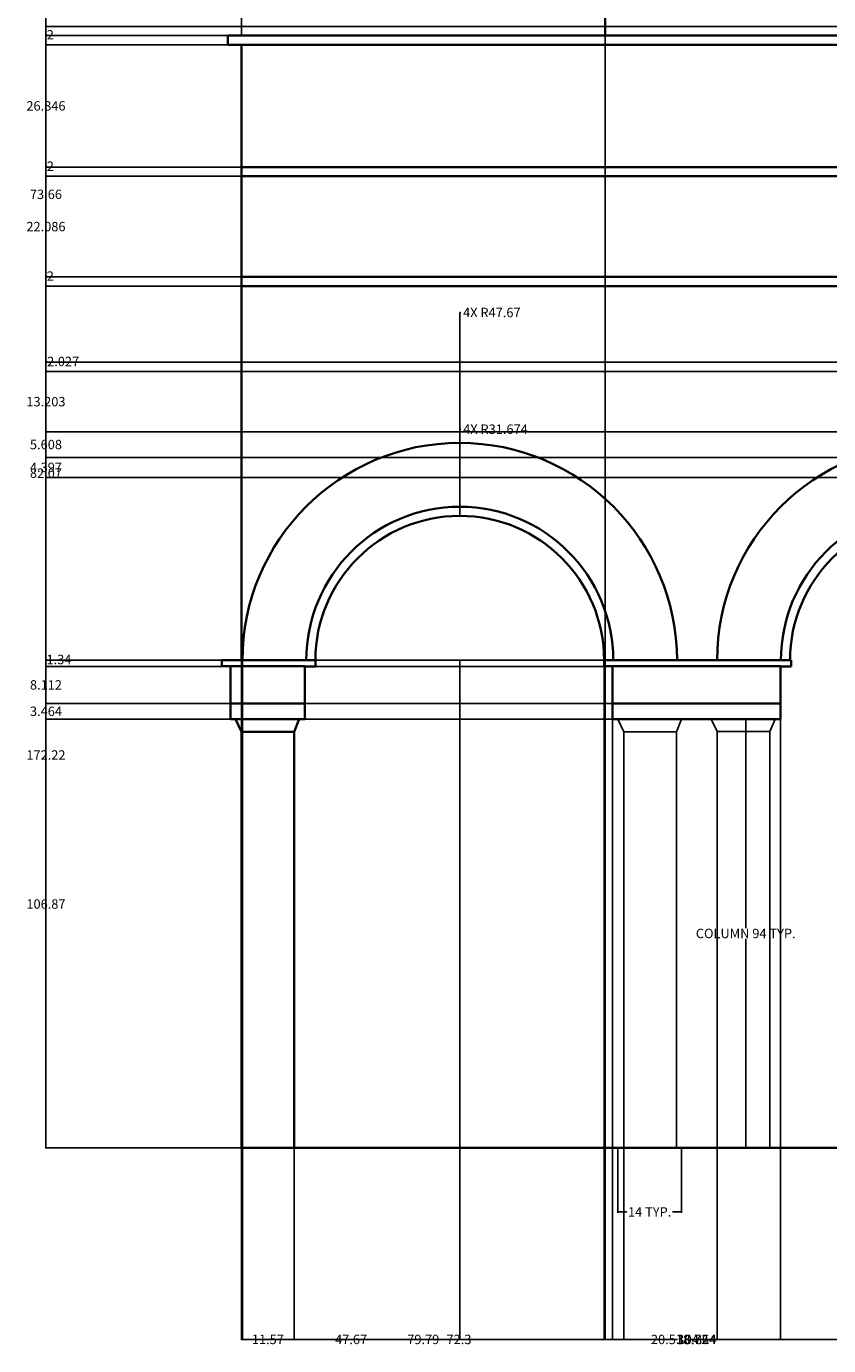
# Model space of a CAD drawing. Units: inches. Extents: x 14 to 859, y 52 to 711.
# Tile 1 of 11: x 14 to 190, y 52 to 342. Entities that reach past the tile are written whole.
import ezdxf

# ---------------------------------------------------------------- set-up
doc = ezdxf.new("R2010")
doc.units = ezdxf.units.IN
doc.header["$MEASUREMENT"] = 0
for name, color, linetype, lineweight in [('A-ANNO-DIMS', 2, 'Continuous', 18), ('A-COLS', 7, 'Continuous', 25), ('A-ELEV', 7, 'Continuous', 35)]:
    doc.layers.add(name, color=color, linetype=linetype, lineweight=lineweight)
doc.styles.get("Standard").update_dxf_attribs({"font": 'arial.ttf'})
doc.dimstyles.get("Standard").update_dxf_attribs({"dimtxt": 2.0625, "dimasz": 0.18, "dimexe": 0.18, "dimexo": 0.0625, "dimgap": 0.09, "dimtad": 0, "dimtih": 1, "dimtoh": 1, "dimdec": 4, "dimzin": 0, "dimdsep": 46, "dimlunit": 4, "dimtxsty": 'Standard', "dimcen": 0.09, "dimadec": 0, "dimazin": 0, "dimtfac": 1, "dimtdec": 4, "dimtofl": 0, "dimtmove": 0, "dimatfit": 3, "dimfxl": 1, "dimtolj": 1, "dimtzin": 0, "dimarcsym": 0})

# ---------------------------------------------------------------- blocks, each defined once
blk = doc.blocks.new('COLUMN')
for p, q in [((1.31, 91.21), (0, 93.94)), ((12.88, 91.21), (13.98, 93.94)), ((1.31, 0), (1.31, 91.21)), ((12.88, 91.21), (1.31, 91.21)), ((12.88, 0), (12.88, 91.21))]:
    blk.add_line(p, q)
blk = doc.blocks.new('*D5')
at = {"layer": 'A-ANNO-DIMS', "color": 0, "lineweight": -2, "transparency": 16777216}
for p, q in [((157.39, 189.73), (171.59, 189.73)), ((171.41, 189.55), (171.41, 143.92)), ((171.41, 95.97), (171.41, 141.6)), ((157.39, 95.79), (171.59, 95.79))]:
    blk.add_line(p, q, dxfattribs=at)
at = {"layer": 'A-ANNO-DIMS', "color": 0, "transparency": 16777216}
for points in [[(171.38, 189.55), (171.44, 189.55), (171.41, 189.73)], [(171.38, 95.97), (171.44, 95.97), (171.41, 95.79)]]:
    blk.add_solid(points, dxfattribs=at)
at = {"layer": 'Defpoints', "color": 0, "transparency": 16777216}
for p in [(157.32, 189.73), (171.41, 189.73), (157.32, 95.79)]:
    blk.add_point(p, dxfattribs=at)
at = {"layer": 'A-ANNO-DIMS', "color": 0, "transparency": 16777216, "insert": (171.41, 142.76), "char_height": 2.0625, "attachment_point": 5}
blk.add_mtext('\\A1;COLUMN 94 TYP.', dxfattribs=at)
blk = doc.blocks.new('*D6')
at = {"layer": 'A-ANNO-DIMS', "color": 0, "lineweight": -2, "transparency": 16777216}
for p, q in [((143.34, 95.73), (143.34, 81.52)), ((157.32, 95.73), (157.32, 81.52)), ((143.52, 81.7), (145.32, 81.7)), ((157.14, 81.7), (155.34, 81.7))]:
    blk.add_line(p, q, dxfattribs=at)
at = {"layer": 'A-ANNO-DIMS', "color": 0, "transparency": 16777216}
for points in [[(143.52, 81.73), (143.52, 81.67), (143.34, 81.7)], [(157.14, 81.73), (157.14, 81.67), (157.32, 81.7)]]:
    blk.add_solid(points, dxfattribs=at)
at = {"layer": 'Defpoints', "color": 0, "transparency": 16777216}
for p in [(143.34, 95.79), (157.32, 95.79), (157.32, 81.7)]:
    blk.add_point(p, dxfattribs=at)
at = {"layer": 'A-ANNO-DIMS', "color": 0, "transparency": 16777216, "insert": (150.33, 81.7), "char_height": 2.0625, "attachment_point": 5}
blk.add_mtext('\\A1;14 TYP.', dxfattribs=at)
blk = doc.blocks.new('*D13')
at = {"layer": 'A-ANNO-DIMS', "color": 0, "lineweight": -2, "transparency": 16777216}
for p, q in [((60.78, 339.73), (60.78, 709.71)), ((60.96, 709.53), (432.6, 709.53)), ((811.37, 709.53), (439.73, 709.53)), ((811.55, 339.73), (811.55, 709.71))]:
    blk.add_line(p, q, dxfattribs=at)
at = {"layer": 'A-ANNO-DIMS', "color": 0, "transparency": 16777216}
for points in [[(60.96, 709.56), (60.96, 709.5), (60.78, 709.53)], [(811.37, 709.56), (811.37, 709.5), (811.55, 709.53)]]:
    blk.add_solid(points, dxfattribs=at)
at = {"layer": 'Defpoints', "color": 0, "transparency": 16777216}
for p in [(811.55, 709.53), (60.78, 339.66), (811.55, 339.66)]:
    blk.add_point(p, dxfattribs=at)
at = {"layer": 'A-ANNO-DIMS', "color": 0, "transparency": 16777216, "insert": (436.17, 709.53), "char_height": 2.062, "attachment_point": 5}
blk.add_mtext('\\A1;750.8', dxfattribs=at)
blk = doc.blocks.new('*D16')
at = {"layer": 'A-ANNO-DIMS', "color": 0, "lineweight": -2, "transparency": 16777216}
for p, q in [((429.96, 670.76), (17.7, 670.76)), ((17.88, 670.58), (17.88, 384.41)), ((17.88, 95.97), (17.88, 382.14)), ((60.72, 95.79), (17.7, 95.79))]:
    blk.add_line(p, q, dxfattribs=at)
at = {"layer": 'A-ANNO-DIMS', "color": 0, "transparency": 16777216}
for points in [[(17.85, 670.58), (17.91, 670.58), (17.88, 670.76)], [(17.85, 95.97), (17.91, 95.97), (17.88, 95.79)]]:
    blk.add_solid(points, dxfattribs=at)
at = {"layer": 'Defpoints', "color": 0, "transparency": 16777216}
for p in [(17.88, 670.76), (430.02, 670.76), (60.78, 95.79)]:
    blk.add_point(p, dxfattribs=at)
at = {"layer": 'A-ANNO-DIMS', "color": 0, "transparency": 16777216, "insert": (17.88, 383.28), "char_height": 2.062, "attachment_point": 5}
blk.add_mtext('\\A1;575', dxfattribs=at)
blk = doc.blocks.new('*D20')
at = {"layer": 'A-ANNO-DIMS', "color": 0, "lineweight": -2, "transparency": 16777216}
for p, q in [((298.67, 268.01), (17.7, 268.01)), ((17.88, 267.83), (17.88, 183.02)), ((17.88, 95.97), (17.88, 180.77)), ((302.61, 95.79), (17.7, 95.79))]:
    blk.add_line(p, q, dxfattribs=at)
at = {"layer": 'A-ANNO-DIMS', "color": 0, "transparency": 16777216}
for points in [[(17.85, 267.83), (17.91, 267.83), (17.88, 268.01)], [(17.85, 95.97), (17.91, 95.97), (17.88, 95.79)]]:
    blk.add_solid(points, dxfattribs=at)
at = {"layer": 'Defpoints', "color": 0, "transparency": 16777216}
for p in [(17.88, 268.01), (298.73, 268.01), (302.67, 95.79)]:
    blk.add_point(p, dxfattribs=at)
at = {"layer": 'A-ANNO-DIMS', "color": 0, "transparency": 16777216, "insert": (17.88, 181.9), "char_height": 2.062, "attachment_point": 5}
blk.add_mtext('\\A1;172.22', dxfattribs=at)
blk = doc.blocks.new('*D25')
at = {"layer": 'A-ANNO-DIMS', "color": 0, "lineweight": -2, "transparency": 16777216}
for p, q in [((298.67, 341.67), (17.7, 341.67)), ((17.88, 341.49), (17.88, 305.98)), ((17.88, 268.19), (17.88, 303.7)), ((298.67, 268.01), (17.7, 268.01))]:
    blk.add_line(p, q, dxfattribs=at)
at = {"layer": 'A-ANNO-DIMS', "color": 0, "transparency": 16777216}
for points in [[(17.85, 341.49), (17.91, 341.49), (17.88, 341.67)], [(17.85, 268.19), (17.91, 268.19), (17.88, 268.01)]]:
    blk.add_solid(points, dxfattribs=at)
at = {"layer": 'Defpoints', "color": 0, "transparency": 16777216}
for p in [(17.88, 341.67), (298.73, 341.67), (298.73, 268.01)]:
    blk.add_point(p, dxfattribs=at)
at = {"layer": 'A-ANNO-DIMS', "color": 0, "transparency": 16777216, "insert": (17.88, 304.84), "char_height": 2.062, "attachment_point": 5}
blk.add_mtext('\\A1;73.66', dxfattribs=at)
blk = doc.blocks.new('*D35')
at = {"layer": 'A-ANNO-DIMS', "color": 0, "lineweight": -2, "transparency": 16777216}
for p, q in [((298.67, 247.17), (17.7, 247.17)), ((17.88, 246.99), (17.88, 246.12)), ((17.88, 242.95), (17.88, 243.83)), ((302.61, 242.77), (17.7, 242.77))]:
    blk.add_line(p, q, dxfattribs=at)
at = {"layer": 'A-ANNO-DIMS', "color": 0, "transparency": 16777216}
for points in [[(17.85, 246.99), (17.91, 246.99), (17.88, 247.17)], [(17.85, 242.95), (17.91, 242.95), (17.88, 242.77)]]:
    blk.add_solid(points, dxfattribs=at)
at = {"layer": 'Defpoints', "color": 0, "transparency": 16777216}
for p in [(17.88, 247.17), (298.73, 247.17), (302.67, 242.77)]:
    blk.add_point(p, dxfattribs=at)
at = {"layer": 'A-ANNO-DIMS', "color": 0, "transparency": 16777216, "insert": (17.88, 244.97), "char_height": 2.062, "attachment_point": 5}
blk.add_mtext('\\A1;4.397', dxfattribs=at)
blk = doc.blocks.new('*D36')
at = {"layer": 'A-ANNO-DIMS', "color": 0, "lineweight": -2, "transparency": 16777216}
for p, q in [((298.67, 252.78), (17.7, 252.78)), ((17.88, 252.6), (17.88, 251.12)), ((17.88, 247.35), (17.88, 248.83)), ((298.67, 247.17), (17.7, 247.17))]:
    blk.add_line(p, q, dxfattribs=at)
at = {"layer": 'A-ANNO-DIMS', "color": 0, "transparency": 16777216}
for points in [[(17.85, 252.6), (17.91, 252.6), (17.88, 252.78)], [(17.85, 247.35), (17.91, 247.35), (17.88, 247.17)]]:
    blk.add_solid(points, dxfattribs=at)
at = {"layer": 'Defpoints', "color": 0, "transparency": 16777216}
for p in [(17.88, 252.78), (298.73, 252.78), (298.73, 247.17)]:
    blk.add_point(p, dxfattribs=at)
at = {"layer": 'A-ANNO-DIMS', "color": 0, "transparency": 16777216, "insert": (17.88, 249.98), "char_height": 2.062, "attachment_point": 5}
blk.add_mtext('\\A1;5.608', dxfattribs=at)
blk = doc.blocks.new('*D37')
at = {"layer": 'A-ANNO-DIMS', "color": 0, "lineweight": -2, "transparency": 16777216}
for p, q in [((298.67, 265.98), (17.7, 265.98)), ((17.88, 265.8), (17.88, 260.53)), ((17.88, 252.96), (17.88, 258.24)), ((298.67, 252.78), (17.7, 252.78))]:
    blk.add_line(p, q, dxfattribs=at)
at = {"layer": 'A-ANNO-DIMS', "color": 0, "transparency": 16777216}
for points in [[(17.85, 265.8), (17.91, 265.8), (17.88, 265.98)], [(17.85, 252.96), (17.91, 252.96), (17.88, 252.78)]]:
    blk.add_solid(points, dxfattribs=at)
at = {"layer": 'Defpoints', "color": 0, "transparency": 16777216}
for p in [(17.88, 265.98), (298.73, 265.98), (298.73, 252.78)]:
    blk.add_point(p, dxfattribs=at)
at = {"layer": 'A-ANNO-DIMS', "color": 0, "transparency": 16777216, "insert": (17.88, 259.38), "char_height": 2.062, "attachment_point": 5}
blk.add_mtext('\\A1;13.203', dxfattribs=at)
blk = doc.blocks.new('*D38')
at = {"layer": 'A-ANNO-DIMS', "color": 0, "lineweight": -2, "transparency": 16777216}
for p, q in [((295.67, 268.01), (17.7, 268.01)), ((17.88, 268.01), (17.88, 268.19)), ((17.88, 268.19), (18.06, 268.19)), ((17.88, 266.16), (17.88, 267.83)), ((295.67, 265.98), (17.7, 265.98))]:
    blk.add_line(p, q, dxfattribs=at)
at = {"layer": 'A-ANNO-DIMS', "color": 0, "transparency": 16777216}
for points in [[(17.85, 267.83), (17.91, 267.83), (17.88, 268.01)], [(17.85, 266.16), (17.91, 266.16), (17.88, 265.98)]]:
    blk.add_solid(points, dxfattribs=at)
at = {"layer": 'Defpoints', "color": 0, "transparency": 16777216}
for p in [(17.88, 268.01), (295.74, 268.01), (295.74, 265.98)]:
    blk.add_point(p, dxfattribs=at)
at = {"layer": 'A-ANNO-DIMS', "color": 0, "transparency": 16777216, "insert": (21.65, 268.19), "char_height": 2.062, "attachment_point": 5}
blk.add_mtext('\\A1;2.027', dxfattribs=at)
blk = doc.blocks.new('*D44')
at = {"layer": 'A-ANNO-DIMS', "color": 0, "lineweight": -2, "transparency": 16777216}
for p, q in [((156.28, 202.66), (17.7, 202.66)), ((17.88, 202.48), (17.88, 150.37)), ((17.88, 95.97), (17.88, 148.08)), ((156.15, 95.79), (17.7, 95.79))]:
    blk.add_line(p, q, dxfattribs=at)
at = {"layer": 'A-ANNO-DIMS', "color": 0, "transparency": 16777216}
for points in [[(17.85, 202.48), (17.91, 202.48), (17.88, 202.66)], [(17.85, 95.97), (17.91, 95.97), (17.88, 95.79)]]:
    blk.add_solid(points, dxfattribs=at)
at = {"layer": 'Defpoints', "color": 0, "transparency": 16777216}
for p in [(17.88, 202.66), (156.35, 202.66), (156.22, 95.79)]:
    blk.add_point(p, dxfattribs=at)
at = {"layer": 'A-ANNO-DIMS', "color": 0, "transparency": 16777216, "insert": (17.88, 149.22), "char_height": 2.062, "attachment_point": 5}
blk.add_mtext('\\A1;106.87', dxfattribs=at)
blk = doc.blocks.new('*D45')
at = {"layer": 'A-ANNO-DIMS', "color": 0, "lineweight": -2, "transparency": 16777216}
for p, q in [((60.78, 95.73), (60.78, 53.56)), ((72.35, 95.73), (72.35, 53.56)), ((60.96, 53.74), (63.09, 53.74)), ((72.17, 53.74), (70.04, 53.74))]:
    blk.add_line(p, q, dxfattribs=at)
at = {"layer": 'A-ANNO-DIMS', "color": 0, "transparency": 16777216}
for points in [[(60.96, 53.77), (60.96, 53.71), (60.78, 53.74)], [(72.17, 53.77), (72.17, 53.71), (72.35, 53.74)]]:
    blk.add_solid(points, dxfattribs=at)
at = {"layer": 'Defpoints', "color": 0, "transparency": 16777216}
for p in [(60.78, 95.79), (72.35, 95.79), (72.35, 53.74)]:
    blk.add_point(p, dxfattribs=at)
at = {"layer": 'A-ANNO-DIMS', "color": 0, "transparency": 16777216, "insert": (66.57, 53.74), "char_height": 2.062, "attachment_point": 5}
blk.add_mtext('\\A1;11.57', dxfattribs=at)
blk = doc.blocks.new('*D46')
at = {"layer": 'A-ANNO-DIMS', "color": 0, "lineweight": -2, "transparency": 16777216}
for p, q in [((72.35, 95.73), (72.35, 53.56)), ((144.65, 95.73), (144.65, 53.56)), ((72.53, 53.74), (105.74, 53.74)), ((144.47, 53.74), (111.26, 53.74))]:
    blk.add_line(p, q, dxfattribs=at)
at = {"layer": 'A-ANNO-DIMS', "color": 0, "transparency": 16777216}
for points in [[(72.53, 53.77), (72.53, 53.71), (72.35, 53.74)], [(144.47, 53.77), (144.47, 53.71), (144.65, 53.74)]]:
    blk.add_solid(points, dxfattribs=at)
at = {"layer": 'Defpoints', "color": 0, "transparency": 16777216}
for p in [(72.35, 95.79), (144.65, 95.79), (144.65, 53.74)]:
    blk.add_point(p, dxfattribs=at)
at = {"layer": 'A-ANNO-DIMS', "color": 0, "transparency": 16777216, "insert": (108.5, 53.74), "char_height": 2.062, "attachment_point": 5}
blk.add_mtext('\\A1;72.3', dxfattribs=at)
blk = doc.blocks.new('*D47')
at = {"layer": 'A-ANNO-DIMS', "color": 0, "lineweight": -2, "transparency": 16777216}
for p, q in [((144.65, 95.73), (144.65, 53.56)), ((165.17, 95.74), (165.17, 53.56)), ((144.83, 53.74), (150.52, 53.74)), ((164.99, 53.74), (159.3, 53.74))]:
    blk.add_line(p, q, dxfattribs=at)
at = {"layer": 'A-ANNO-DIMS', "color": 0, "transparency": 16777216}
for points in [[(144.83, 53.77), (144.83, 53.71), (144.65, 53.74)], [(164.99, 53.77), (164.99, 53.71), (165.17, 53.74)]]:
    blk.add_solid(points, dxfattribs=at)
at = {"layer": 'Defpoints', "color": 0, "transparency": 16777216}
for p in [(144.65, 95.79), (165.17, 95.8), (165.17, 53.74)]:
    blk.add_point(p, dxfattribs=at)
at = {"layer": 'A-ANNO-DIMS', "color": 0, "transparency": 16777216, "insert": (154.91, 53.74), "char_height": 2.062, "attachment_point": 5}
blk.add_mtext('\\A1;20.518', dxfattribs=at)
blk = doc.blocks.new('*D48')
at = {"layer": 'A-ANNO-DIMS', "color": 0, "lineweight": -2, "transparency": 16777216}
for p, q in [((165.17, 95.74), (165.17, 53.56)), ((247.79, 95.73), (247.79, 53.56)), ((165.35, 53.74), (202.92, 53.74)), ((247.61, 53.74), (210.04, 53.74))]:
    blk.add_line(p, q, dxfattribs=at)
at = {"layer": 'A-ANNO-DIMS', "color": 0, "transparency": 16777216}
for points in [[(165.35, 53.77), (165.35, 53.71), (165.17, 53.74)], [(247.61, 53.77), (247.61, 53.71), (247.79, 53.74)]]:
    blk.add_solid(points, dxfattribs=at)
at = {"layer": 'Defpoints', "color": 0, "transparency": 16777216}
for p in [(165.17, 95.8), (247.79, 95.79), (247.79, 53.74)]:
    blk.add_point(p, dxfattribs=at)
at = {"layer": 'A-ANNO-DIMS', "color": 0, "transparency": 16777216, "insert": (206.48, 53.74), "char_height": 2.062, "attachment_point": 5}
blk.add_mtext('\\A1;82.62', dxfattribs=at)
blk = doc.blocks.new('*D50')
at = {"layer": 'A-ANNO-DIMS', "color": 0, "lineweight": -2, "transparency": 16777216}
for p, q in [((61, 202.6), (61, 53.56)), ((108.67, 202.6), (108.67, 53.56)), ((61.18, 53.74), (81.22, 53.74)), ((108.49, 53.74), (88.45, 53.74))]:
    blk.add_line(p, q, dxfattribs=at)
at = {"layer": 'A-ANNO-DIMS', "color": 0, "transparency": 16777216}
for points in [[(61.18, 53.77), (61.18, 53.71), (61, 53.74)], [(108.49, 53.77), (108.49, 53.71), (108.67, 53.74)]]:
    blk.add_solid(points, dxfattribs=at)
at = {"layer": 'Defpoints', "color": 0, "transparency": 16777216}
for p in [(61, 202.66), (108.67, 202.66), (108.67, 53.74)]:
    blk.add_point(p, dxfattribs=at)
at = {"layer": 'A-ANNO-DIMS', "color": 0, "transparency": 16777216, "insert": (84.83, 53.74), "char_height": 2.062, "attachment_point": 5}
blk.add_mtext('\\A1;47.67', dxfattribs=at)
blk = doc.blocks.new('*D51')
at = {"layer": 'A-ANNO-DIMS', "color": 0, "lineweight": -2, "transparency": 16777216}
for p, q in [((108.67, 202.6), (108.67, 53.56)), ((212.81, 202.6), (212.81, 53.56)), ((108.85, 53.74), (156.47, 53.74)), ((212.63, 53.74), (165.01, 53.74))]:
    blk.add_line(p, q, dxfattribs=at)
at = {"layer": 'A-ANNO-DIMS', "color": 0, "transparency": 16777216}
for points in [[(108.85, 53.77), (108.85, 53.71), (108.67, 53.74)], [(212.63, 53.77), (212.63, 53.71), (212.81, 53.74)]]:
    blk.add_solid(points, dxfattribs=at)
at = {"layer": 'Defpoints', "color": 0, "transparency": 16777216}
for p in [(108.67, 202.66), (212.81, 202.66), (212.81, 53.74)]:
    blk.add_point(p, dxfattribs=at)
at = {"layer": 'A-ANNO-DIMS', "color": 0, "transparency": 16777216, "insert": (160.74, 53.74), "char_height": 2.062, "attachment_point": 5}
blk.add_mtext('\\A1;104.14', dxfattribs=at)
blk = doc.blocks.new('*D53')
at = {"layer": 'A-ANNO-DIMS', "color": 0, "lineweight": -2, "transparency": 16777216}
for p, q in [((60.72, 284.73), (17.7, 284.73)), ((17.88, 284.55), (17.88, 244.84)), ((17.88, 202.84), (17.88, 242.55)), ((60.93, 202.66), (17.7, 202.66))]:
    blk.add_line(p, q, dxfattribs=at)
at = {"layer": 'A-ANNO-DIMS', "color": 0, "transparency": 16777216}
for points in [[(17.85, 284.55), (17.91, 284.55), (17.88, 284.73)], [(17.85, 202.84), (17.91, 202.84), (17.88, 202.66)]]:
    blk.add_solid(points, dxfattribs=at)
at = {"layer": 'Defpoints', "color": 0, "transparency": 16777216}
for p in [(17.88, 284.73), (60.78, 284.73), (61, 202.66)]:
    blk.add_point(p, dxfattribs=at)
at = {"layer": 'A-ANNO-DIMS', "color": 0, "transparency": 16777216, "insert": (17.88, 243.7), "char_height": 2.062, "attachment_point": 5}
blk.add_mtext('\\A1;82.07', dxfattribs=at)
blk = doc.blocks.new('*D54')
at = {"layer": 'A-ANNO-DIMS', "color": 0, "lineweight": -2, "transparency": 16777216}
for p, q in [((60.72, 286.73), (17.7, 286.73)), ((17.88, 286.73), (17.88, 286.91)), ((17.88, 286.91), (18.06, 286.91)), ((17.88, 284.91), (17.88, 286.55)), ((60.72, 284.73), (17.7, 284.73))]:
    blk.add_line(p, q, dxfattribs=at)
at = {"layer": 'A-ANNO-DIMS', "color": 0, "transparency": 16777216}
for points in [[(17.85, 286.55), (17.91, 286.55), (17.88, 286.73)], [(17.85, 284.91), (17.91, 284.91), (17.88, 284.73)]]:
    blk.add_solid(points, dxfattribs=at)
at = {"layer": 'Defpoints', "color": 0, "transparency": 16777216}
for p in [(17.88, 286.73), (60.78, 286.73), (60.78, 284.73)]:
    blk.add_point(p, dxfattribs=at)
at = {"layer": 'A-ANNO-DIMS', "color": 0, "transparency": 16777216, "insert": (18.83, 286.91), "char_height": 2.062, "attachment_point": 5}
blk.add_mtext('\\A1;2', dxfattribs=at)
blk = doc.blocks.new('*D55')
at = {"layer": 'A-ANNO-DIMS', "color": 0, "lineweight": -2, "transparency": 16777216}
for p, q in [((60.72, 308.82), (17.7, 308.82)), ((17.88, 308.64), (17.88, 298.92)), ((17.88, 286.91), (17.88, 296.63)), ((60.72, 286.73), (17.7, 286.73))]:
    blk.add_line(p, q, dxfattribs=at)
at = {"layer": 'A-ANNO-DIMS', "color": 0, "transparency": 16777216}
for points in [[(17.85, 308.64), (17.91, 308.64), (17.88, 308.82)], [(17.85, 286.91), (17.91, 286.91), (17.88, 286.73)]]:
    blk.add_solid(points, dxfattribs=at)
at = {"layer": 'Defpoints', "color": 0, "transparency": 16777216}
for p in [(17.88, 308.82), (60.78, 308.82), (60.78, 286.73)]:
    blk.add_point(p, dxfattribs=at)
at = {"layer": 'A-ANNO-DIMS', "color": 0, "transparency": 16777216, "insert": (17.88, 297.77), "char_height": 2.062, "attachment_point": 5}
blk.add_mtext('\\A1;22.086', dxfattribs=at)
blk = doc.blocks.new('*D56')
at = {"layer": 'A-ANNO-DIMS', "color": 0, "lineweight": -2, "transparency": 16777216}
for p, q in [((60.72, 310.82), (17.7, 310.82)), ((17.88, 310.82), (17.88, 311)), ((17.88, 311), (18.06, 311)), ((17.88, 309), (17.88, 310.64)), ((60.72, 308.82), (17.7, 308.82))]:
    blk.add_line(p, q, dxfattribs=at)
at = {"layer": 'A-ANNO-DIMS', "color": 0, "transparency": 16777216}
for points in [[(17.85, 310.64), (17.91, 310.64), (17.88, 310.82)], [(17.85, 309), (17.91, 309), (17.88, 308.82)]]:
    blk.add_solid(points, dxfattribs=at)
at = {"layer": 'Defpoints', "color": 0, "transparency": 16777216}
for p in [(17.88, 310.82), (60.78, 310.82), (60.78, 308.82)]:
    blk.add_point(p, dxfattribs=at)
at = {"layer": 'A-ANNO-DIMS', "color": 0, "transparency": 16777216, "insert": (18.83, 311), "char_height": 2.062, "attachment_point": 5}
blk.add_mtext('\\A1;2', dxfattribs=at)
blk = doc.blocks.new('*D57')
at = {"layer": 'A-ANNO-DIMS', "color": 0, "lineweight": -2, "transparency": 16777216}
for p, q in [((60.72, 337.66), (17.7, 337.66)), ((17.88, 337.48), (17.88, 325.38)), ((17.88, 311), (17.88, 323.1)), ((60.72, 310.82), (17.7, 310.82))]:
    blk.add_line(p, q, dxfattribs=at)
at = {"layer": 'A-ANNO-DIMS', "color": 0, "transparency": 16777216}
for points in [[(17.85, 337.48), (17.91, 337.48), (17.88, 337.66)], [(17.85, 311), (17.91, 311), (17.88, 310.82)]]:
    blk.add_solid(points, dxfattribs=at)
at = {"layer": 'Defpoints', "color": 0, "transparency": 16777216}
for p in [(17.88, 337.66), (60.78, 337.66), (60.78, 310.82)]:
    blk.add_point(p, dxfattribs=at)
at = {"layer": 'A-ANNO-DIMS', "color": 0, "transparency": 16777216, "insert": (17.88, 324.24), "char_height": 2.062, "attachment_point": 5}
blk.add_mtext('\\A1;26.846', dxfattribs=at)
blk = doc.blocks.new('*D58')
at = {"layer": 'A-ANNO-DIMS', "color": 0, "lineweight": -2, "transparency": 16777216}
for p, q in [((60.72, 339.66), (17.7, 339.66)), ((17.88, 339.66), (17.88, 339.84)), ((17.88, 339.84), (18.06, 339.84)), ((17.88, 337.84), (17.88, 339.48)), ((60.72, 337.66), (17.7, 337.66))]:
    blk.add_line(p, q, dxfattribs=at)
at = {"layer": 'A-ANNO-DIMS', "color": 0, "transparency": 16777216}
for points in [[(17.85, 339.48), (17.91, 339.48), (17.88, 339.66)], [(17.85, 337.84), (17.91, 337.84), (17.88, 337.66)]]:
    blk.add_solid(points, dxfattribs=at)
at = {"layer": 'Defpoints', "color": 0, "transparency": 16777216}
for p in [(17.88, 339.66), (60.78, 339.66), (60.78, 337.66)]:
    blk.add_point(p, dxfattribs=at)
at = {"layer": 'A-ANNO-DIMS', "color": 0, "transparency": 16777216, "insert": (18.83, 339.84), "char_height": 2.062, "attachment_point": 5}
blk.add_mtext('\\A1;2', dxfattribs=at)
blk = doc.blocks.new('*D59')
at = {"layer": 'A-ANNO-DIMS', "color": 0, "lineweight": -2, "transparency": 16777216}
for p, q in [((140.51, 404.37), (17.7, 404.37)), ((17.88, 404.19), (17.88, 373.16)), ((17.88, 339.84), (17.88, 370.87)), ((140.51, 339.66), (17.7, 339.66))]:
    blk.add_line(p, q, dxfattribs=at)
at = {"layer": 'A-ANNO-DIMS', "color": 0, "transparency": 16777216}
for points in [[(17.85, 404.19), (17.91, 404.19), (17.88, 404.37)], [(17.85, 339.84), (17.91, 339.84), (17.88, 339.66)]]:
    blk.add_solid(points, dxfattribs=at)
at = {"layer": 'Defpoints', "color": 0, "transparency": 16777216}
for p in [(17.88, 404.37), (140.57, 404.37), (140.57, 339.66)]:
    blk.add_point(p, dxfattribs=at)
at = {"layer": 'A-ANNO-DIMS', "color": 0, "transparency": 16777216, "insert": (17.88, 372.02), "char_height": 2.062, "attachment_point": 5}
blk.add_mtext('\\A1;64.71', dxfattribs=at)
blk = doc.blocks.new('*D61')
at = {"layer": 'A-ANNO-DIMS', "color": 0, "lineweight": -2, "transparency": 16777216}
for p, q in [((140.57, 339.6), (140.57, 53.56)), ((60.78, 337.6), (60.78, 53.56)), ((60.96, 53.74), (97.11, 53.74)), ((140.39, 53.74), (104.24, 53.74))]:
    blk.add_line(p, q, dxfattribs=at)
at = {"layer": 'A-ANNO-DIMS', "color": 0, "transparency": 16777216}
for points in [[(60.96, 53.77), (60.96, 53.71), (60.78, 53.74)], [(140.39, 53.77), (140.39, 53.71), (140.57, 53.74)]]:
    blk.add_solid(points, dxfattribs=at)
at = {"layer": 'Defpoints', "color": 0, "transparency": 16777216}
for p in [(140.57, 339.66), (60.78, 337.66), (140.57, 53.74)]:
    blk.add_point(p, dxfattribs=at)
at = {"layer": 'A-ANNO-DIMS', "color": 0, "transparency": 16777216, "insert": (100.67, 53.74), "char_height": 2.062, "attachment_point": 5}
blk.add_mtext('\\A1;79.79', dxfattribs=at)
blk = doc.blocks.new('*D68')
at = {"layer": 'A-ANNO-DIMS', "color": 0, "lineweight": -2, "transparency": 16777216}
for p, q in [((179, 193.21), (17.7, 193.21)), ((17.88, 193.03), (17.88, 192.62)), ((177.78, 189.74), (17.7, 189.74)), ((17.88, 189.92), (17.88, 190.33))]:
    blk.add_line(p, q, dxfattribs=at)
at = {"layer": 'A-ANNO-DIMS', "color": 0, "transparency": 16777216}
for points in [[(17.85, 193.03), (17.91, 193.03), (17.88, 193.21)], [(17.85, 189.92), (17.91, 189.92), (17.88, 189.74)]]:
    blk.add_solid(points, dxfattribs=at)
at = {"layer": 'Defpoints', "color": 0, "transparency": 16777216}
for p in [(17.88, 193.21), (179.07, 193.21), (177.84, 189.74)]:
    blk.add_point(p, dxfattribs=at)
at = {"layer": 'A-ANNO-DIMS', "color": 0, "transparency": 16777216, "insert": (17.88, 191.48), "char_height": 2.062, "attachment_point": 5}
blk.add_mtext('\\A1;3.464', dxfattribs=at)
blk = doc.blocks.new('*D69')
at = {"layer": 'A-ANNO-DIMS', "color": 0, "lineweight": -2, "transparency": 16777216}
for p, q in [((179, 201.32), (17.7, 201.32)), ((17.88, 201.14), (17.88, 198.41)), ((17.88, 193.39), (17.88, 196.12)), ((179, 193.21), (17.7, 193.21))]:
    blk.add_line(p, q, dxfattribs=at)
at = {"layer": 'A-ANNO-DIMS', "color": 0, "transparency": 16777216}
for points in [[(17.85, 201.14), (17.91, 201.14), (17.88, 201.32)], [(17.85, 193.39), (17.91, 193.39), (17.88, 193.21)]]:
    blk.add_solid(points, dxfattribs=at)
at = {"layer": 'Defpoints', "color": 0, "transparency": 16777216}
for p in [(17.88, 201.32), (179.07, 201.32), (179.07, 193.21)]:
    blk.add_point(p, dxfattribs=at)
at = {"layer": 'A-ANNO-DIMS', "color": 0, "transparency": 16777216, "insert": (17.88, 197.27), "char_height": 2.062, "attachment_point": 5}
blk.add_mtext('\\A1;8.112', dxfattribs=at)
blk = doc.blocks.new('*D70')
at = {"layer": 'A-ANNO-DIMS', "color": 0, "lineweight": -2, "transparency": 16777216}
for p, q in [((179.07, 202.66), (17.7, 202.66)), ((17.88, 202.66), (17.88, 202.84)), ((17.88, 202.84), (18.06, 202.84)), ((179, 201.32), (17.7, 201.32)), ((17.88, 201.5), (17.88, 202.48))]:
    blk.add_line(p, q, dxfattribs=at)
at = {"layer": 'A-ANNO-DIMS', "color": 0, "transparency": 16777216}
for points in [[(17.85, 202.48), (17.91, 202.48), (17.88, 202.66)], [(17.85, 201.5), (17.91, 201.5), (17.88, 201.32)]]:
    blk.add_solid(points, dxfattribs=at)
at = {"layer": 'Defpoints', "color": 0, "transparency": 16777216}
for p in [(17.88, 202.66), (179.14, 202.66), (179.07, 201.32)]:
    blk.add_point(p, dxfattribs=at)
at = {"layer": 'A-ANNO-DIMS', "color": 0, "transparency": 16777216, "insert": (20.73, 202.84), "char_height": 2.062, "attachment_point": 5}
blk.add_mtext('\\A1;1.34', dxfattribs=at)
blk = doc.blocks.new('*D71')
at = {"layer": 'A-ANNO-DIMS', "color": 0, "lineweight": -2, "transparency": 16777216}
for p, q in [((142.2, 193.15), (142.2, 53.56)), ((179.07, 193.15), (179.07, 53.56)), ((142.38, 53.74), (156.27, 53.74)), ((178.89, 53.74), (165, 53.74))]:
    blk.add_line(p, q, dxfattribs=at)
at = {"layer": 'A-ANNO-DIMS', "color": 0, "transparency": 16777216}
for points in [[(142.38, 53.77), (142.38, 53.71), (142.2, 53.74)], [(178.89, 53.77), (178.89, 53.71), (179.07, 53.74)]]:
    blk.add_solid(points, dxfattribs=at)
at = {"layer": 'Defpoints', "color": 0, "transparency": 16777216}
for p in [(142.2, 193.21), (179.07, 193.21), (179.07, 53.74)]:
    blk.add_point(p, dxfattribs=at)
at = {"layer": 'A-ANNO-DIMS', "color": 0, "transparency": 16777216, "insert": (160.63, 53.74), "char_height": 2.062, "attachment_point": 5}
blk.add_mtext('\\A1;36.864', dxfattribs=at)
blk = doc.blocks.new('*D72')
at = {"layer": 'A-ANNO-DIMS', "color": 0, "lineweight": -2, "transparency": 16777216}
for p, q in [((140.35, 201.34), (140.35, 53.56)), ((179.07, 201.26), (179.07, 53.56)), ((140.53, 53.74), (156.15, 53.74)), ((178.89, 53.74), (163.26, 53.74))]:
    blk.add_line(p, q, dxfattribs=at)
at = {"layer": 'A-ANNO-DIMS', "color": 0, "transparency": 16777216}
for points in [[(140.53, 53.77), (140.53, 53.71), (140.35, 53.74)], [(178.89, 53.77), (178.89, 53.71), (179.07, 53.74)]]:
    blk.add_solid(points, dxfattribs=at)
at = {"layer": 'Defpoints', "color": 0, "transparency": 16777216}
for p in [(140.35, 201.4), (179.07, 201.32), (179.07, 53.74)]:
    blk.add_point(p, dxfattribs=at)
at = {"layer": 'A-ANNO-DIMS', "color": 0, "transparency": 16777216, "insert": (159.71, 53.74), "char_height": 2.062, "attachment_point": 5}
blk.add_mtext('\\A1;38.72', dxfattribs=at)
blk = doc.blocks.new('*D127')
at = {"layer": 'A-ANNO-DIMS', "color": 0, "lineweight": -2, "transparency": 16777216}
for p, q in [((108.72, 278.94), (108.7, 250.51)), ((108.9, 278.94), (108.72, 278.94)), ((108.58, 202.66), (108.76, 202.66)), ((108.67, 202.57), (108.67, 202.75))]:
    blk.add_line(p, q, dxfattribs=at)
at = {"layer": 'A-ANNO-DIMS', "color": 0, "transparency": 16777216}
blk.add_solid([(108.67, 250.51), (108.73, 250.51), (108.7, 250.33)], dxfattribs=at)
at = {"layer": 'Defpoints', "color": 0, "transparency": 16777216}
for p in [(108.7, 250.33), (108.67, 202.66)]:
    blk.add_point(p, dxfattribs=at)
at = {"layer": 'A-ANNO-DIMS', "color": 0, "transparency": 16777216, "insert": (115.71, 278.94), "char_height": 2.0625, "attachment_point": 5}
blk.add_mtext('\\A1;4X R47.67', dxfattribs=at)
blk = doc.blocks.new('*D129')
at = {"layer": 'A-ANNO-DIMS', "color": 0, "lineweight": -2, "transparency": 16777216}
for p, q in [((108.72, 253.34), (108.7, 234.51)), ((108.9, 253.34), (108.72, 253.34)), ((108.58, 202.66), (108.76, 202.66)), ((108.67, 202.57), (108.67, 202.75))]:
    blk.add_line(p, q, dxfattribs=at)
at = {"layer": 'A-ANNO-DIMS', "color": 0, "transparency": 16777216}
blk.add_solid([(108.67, 234.51), (108.73, 234.51), (108.7, 234.33)], dxfattribs=at)
at = {"layer": 'Defpoints', "color": 0, "transparency": 16777216}
for p in [(108.7, 234.33), (108.67, 202.66)]:
    blk.add_point(p, dxfattribs=at)
at = {"layer": 'A-ANNO-DIMS', "color": 0, "transparency": 16777216, "insert": (116.51, 253.34), "char_height": 2.0625, "attachment_point": 5}
blk.add_mtext('\\A1;4X R31.674', dxfattribs=at)

msp = doc.modelspace()

# ---------------------------------------------------------------- linework, layer by layer
at = {"layer": 'A-ELEV'}
for p, q in [((140.5683, 339.6626), (140.5683, 404.3712)), ((60.7804, 339.6626), (57.8159, 339.6626)), ((57.8159, 339.6626), (57.8159, 337.6626)), ((60.7804, 339.6626), (262.6537, 339.6626)), ((57.8159, 337.6626), (60.7804, 337.6626)), ((60.7804, 303.3146), (60.7804, 337.6626)), ((60.7804, 337.6626), (262.6537, 337.6626)), ((60.7804, 310.8171), (262.6537, 310.8171)), ((60.7804, 308.8171), (262.6537, 308.8171)), ((60.7804, 263.7876), (60.7804, 303.3146)), ((60.7804, 286.7316), (262.6537, 286.7316)), ((60.7804, 284.7316), (262.6537, 284.7316)), ((60.7804, 202.6598), (60.7804, 263.7876)), ((56.4785, 201.4021), (56.4785, 202.6598)), ((56.4785, 202.6598), (76.9974, 202.6598)), ((76.9974, 202.6598), (76.9974, 201.3212)), ((140.3457, 201.4021), (140.3457, 202.6598)), ((140.3457, 202.6598), (160.8646, 202.6598)), ((160.8646, 202.6598), (181.3835, 202.6598)), ((181.3835, 202.6598), (181.3835, 201.3212)), ((58.3352, 201.4021), (56.4785, 201.4021)), ((58.3352, 193.2091), (58.3352, 201.4021)), ((58.3352, 201.4021), (74.68, 201.4021)), ((74.68, 201.4021), (74.68, 193.2091)), ((76.9974, 201.3212), (74.68, 201.3212)), ((142.2024, 201.4021), (140.3457, 201.4021)), ((142.2024, 193.2091), (142.2024, 201.4021)), ((142.2024, 201.4021), (158.5472, 201.4021)), ((158.5472, 201.4021), (160.8646, 201.4021)), ((162.7213, 201.4021), (160.8646, 201.4021)), ((162.7213, 201.4021), (179.0661, 201.4021)), ((179.0661, 201.4021), (179.0661, 193.2091)), ((181.3835, 201.3212), (179.0661, 201.3212)), ((58.3352, 189.7289), (58.3352, 193.2091)), ((58.3352, 193.2091), (74.68, 193.2091)), ((74.68, 193.2091), (74.68, 189.7289)), ((142.2024, 189.7289), (142.2024, 193.2091)), ((142.2024, 193.2091), (158.5472, 193.2091)), ((158.5472, 193.2091), (162.7213, 193.2091)), ((162.7213, 193.2091), (179.0661, 193.2091)), ((179.0661, 193.2091), (179.0661, 189.7289)), ((74.68, 189.7289), (58.3352, 189.7289)), ((60.7804, 187.0003), (59.4726, 189.7289)), ((72.3501, 187.0003), (73.4563, 189.7289)), ((158.5472, 189.7289), (142.2024, 189.7289)), ((158.5472, 189.7289), (162.7213, 189.7289)), ((179.0661, 189.7289), (162.7213, 189.7289)), ((60.7804, 95.7876), (60.7804, 187.0003)), ((72.3501, 187.0003), (60.7804, 187.0003)), ((72.3501, 95.7876), (72.3501, 187.0003)), ((60.7804, 95.7876), (262.6537, 95.7876))]:
    msp.add_line(p, q, dxfattribs=at)
for centre, radius in [((108.6715, 202.6598), 47.6742), ((212.8108, 202.6598), 47.6742), ((108.6715, 202.6598), 33.6742), ((108.6715, 202.6598), 31.6742), ((212.8108, 202.6598), 33.6742), ((212.8108, 202.6598), 31.6742)]:
    msp.add_arc(centre, radius, 0, 180, dxfattribs=at)

# ---------------------------------------------------------------- block references
at = {"layer": 'A-COLS'}
msp.add_blockref('COLUMN', (143.34, 95.788), dxfattribs=at)
at = {"layer": 'A-COLS', "rotation": 359.9990108211547}
msp.add_blockref('COLUMN', (163.8576, 95.8043), dxfattribs=at)

# ---------------------------------------------------------------- dimensions: what is measured, and where the dimension line sits
at = {"layer": 'A-ANNO-DIMS'}
for base, p1, p2, override, picture, middle in [((811.5534, 709.5262), (60.7804, 339.6626), (811.5534, 339.6626), {"dimdec": 1, "dimlfac": 1, "dimrnd": 0, "dimzin": 0, "dimdsep": 46, "dimlunit": 2}, '*D13', (436.1669, 709.5262)), ((140.5683, 53.7364), (60.7804, 337.6626), (140.5683, 339.6626), {"dimdec": 2, "dimlfac": 1, "dimrnd": 0, "dimzin": 0, "dimdsep": 46, "dimlunit": 2}, '*D61', (100.6744, 53.7364)), ((108.6715, 53.7364), (60.9974, 202.6598), (108.6715, 202.6598), {"dimdec": 2, "dimlfac": 1, "dimrnd": 0, "dimzin": 0, "dimdsep": 46, "dimlunit": 2}, '*D50', (84.8345, 53.7364)), ((212.8108, 53.7364), (108.6715, 202.6598), (212.8108, 202.6598), {"dimdec": 2, "dimlfac": 1, "dimrnd": 0, "dimzin": 0, "dimdsep": 46, "dimlunit": 2}, '*D51', (160.7412, 53.7364)), ((179.0661, 53.7364), (140.3457, 201.4021), (179.0661, 201.3212), {"dimdec": 2, "dimlfac": 1, "dimrnd": 0, "dimzin": 0, "dimdsep": 46, "dimlunit": 2}, '*D72', (159.7059, 53.7364)), ((179.0661, 53.7364), (142.2024, 193.2091), (179.0661, 193.2091), {"dimdec": 3, "dimlfac": 1, "dimrnd": 0, "dimzin": 0, "dimdsep": 46, "dimlunit": 2}, '*D71', (160.6343, 53.7364)), ((72.3501, 53.7364), (60.7804, 95.7876), (72.3501, 95.7876), {"dimdec": 2, "dimlfac": 1, "dimrnd": 0, "dimzin": 0, "dimdsep": 46, "dimlunit": 2}, '*D45', (66.5652, 53.7364)), ((144.6476, 53.7364), (72.3501, 95.7876), (144.6476, 95.7876), {"dimdec": 1, "dimlfac": 1, "dimrnd": 0, "dimzin": 0, "dimdsep": 46, "dimlunit": 2}, '*D46', (108.4988, 53.7364)), ((165.1652, 53.7364), (144.6476, 95.7876), (165.1652, 95.8039), {"dimdec": 3, "dimlfac": 1, "dimrnd": 0, "dimzin": 0, "dimdsep": 46, "dimlunit": 2}, '*D47', (154.9064, 53.7364)), ((247.7877, 53.7364), (165.1652, 95.8039), (247.7877, 95.7876), {"dimdec": 2, "dimlfac": 1, "dimrnd": 0, "dimzin": 0, "dimdsep": 46, "dimlunit": 2}, '*D48', (206.4765, 53.7364))]:
    dim = msp.add_linear_dim(base=base, p1=p1, p2=p2, dimstyle='Standard', override=override, dxfattribs=at)
    dim.commit()
    dim.dimension.update_dxf_attribs({"geometry": picture, "text_midpoint": middle})
for base, p1, p2, override, picture, middle in [((17.8785, 670.7637), (60.7804, 95.7876), (430.0228, 670.7637), {"dimdec": 0, "dimlfac": 1, "dimrnd": 0, "dimzin": 0, "dimdsep": 46, "dimlunit": 2}, '*D16', (17.8785, 383.2756)), ((17.8785, 404.3712), (140.5683, 339.6626), (140.5683, 404.3712), {"dimdec": 2, "dimlfac": 1, "dimrnd": 0, "dimzin": 0, "dimdsep": 46, "dimlunit": 2}, '*D59', (17.8785, 372.0169)), ((17.8785, 341.6716), (298.7295, 268.0097), (298.7295, 341.6716), {"dimdec": 2, "dimlfac": 1, "dimrnd": 0, "dimzin": 0, "dimdsep": 46, "dimlunit": 2}, '*D25', (17.8785, 304.8406)), ((17.8785, 339.6626), (60.7804, 337.6626), (60.7804, 339.6626), {"dimdec": 0, "dimlfac": 1, "dimrnd": 0, "dimzin": 0, "dimdsep": 46, "dimlunit": 2}, '*D58', (18.8315, 339.8426)), ((17.87849, 337.66265), (60.7804, 310.81712), (60.7804, 337.66265), {"dimdec": 3, "dimlfac": 1, "dimrnd": 0, "dimzin": 0, "dimdsep": 46, "dimlunit": 2}, '*D57', (17.87849, 324.23989)), ((17.8785, 310.8171), (60.7804, 308.8171), (60.7804, 310.8171), {"dimdec": 0, "dimlfac": 1, "dimrnd": 0, "dimzin": 0, "dimdsep": 46, "dimlunit": 2}, '*D56', (18.8315, 310.9971)), ((17.87849, 308.81712), (60.7804, 286.73158), (60.7804, 308.81712), {"dimdec": 3, "dimlfac": 1, "dimrnd": 0, "dimzin": 0, "dimdsep": 46, "dimlunit": 2}, '*D55', (17.87849, 297.77435)), ((17.8785, 286.7316), (60.7804, 284.7316), (60.7804, 286.7316), {"dimdec": 0, "dimlfac": 1, "dimrnd": 0, "dimzin": 0, "dimdsep": 46, "dimlunit": 2}, '*D54', (18.8315, 286.9116)), ((17.8785, 284.7316), (60.9974, 202.6598), (60.7804, 284.7316), {"dimdec": 2, "dimlfac": 1, "dimrnd": 0, "dimzin": 0, "dimdsep": 46, "dimlunit": 2}, '*D53', (17.8785, 243.6957)), ((17.8785, 268.0097), (295.7375, 265.9828), (295.7375, 268.0097), {"dimdec": 3, "dimlfac": 1, "dimrnd": 0, "dimzin": 0, "dimdsep": 46, "dimlunit": 2}, '*D38', (21.646, 268.1897)), ((17.8785, 268.0097), (302.6699, 95.7876), (298.7295, 268.0097), {"dimdec": 2, "dimlfac": 1, "dimrnd": 0, "dimzin": 0, "dimdsep": 46, "dimlunit": 2}, '*D20', (17.8785, 181.8987)), ((17.8785, 265.9828), (298.7295, 252.7801), (298.7295, 265.9828), {"dimdec": 3, "dimlfac": 1, "dimrnd": 0, "dimzin": 0, "dimdsep": 46, "dimlunit": 2}, '*D37', (17.8785, 259.3815)), ((17.8785, 252.7801), (298.7295, 247.1718), (298.7295, 252.7801), {"dimdec": 3, "dimlfac": 1, "dimrnd": 0, "dimzin": 0, "dimdsep": 46, "dimlunit": 2}, '*D36', (17.8785, 249.9759)), ((17.8785, 247.1718), (302.6699, 242.7747), (298.7295, 247.1718), {"dimdec": 3, "dimlfac": 1, "dimrnd": 0, "dimzin": 0, "dimdsep": 46, "dimlunit": 2}, '*D35', (17.8785, 244.9732)), ((17.8785, 202.6598), (156.2173, 95.7876), (156.3457, 202.6598), {"dimdec": 2, "dimlfac": 1, "dimrnd": 0, "dimzin": 0, "dimdsep": 46, "dimlunit": 2}, '*D44', (17.8785, 149.2237)), ((17.8785, 202.6598), (179.0661, 201.3212), (179.1366, 202.6598), {"dimdec": 2, "dimlfac": 1, "dimrnd": 0, "dimzin": 0, "dimdsep": 46, "dimlunit": 2}, '*D70', (20.7259, 202.8398)), ((17.8785, 201.3212), (179.0661, 193.2091), (179.0661, 201.3212), {"dimdec": 3, "dimlfac": 1, "dimrnd": 0, "dimzin": 0, "dimdsep": 46, "dimlunit": 2}, '*D69', (17.8785, 197.2652)), ((17.8785, 193.2091), (177.8428, 189.7449), (179.0661, 193.2091), {"dimdec": 3, "dimlfac": 1, "dimrnd": 0, "dimzin": 0, "dimdsep": 46, "dimlunit": 2}, '*D68', (17.8785, 191.477))]:
    dim = msp.add_linear_dim(base=base, p1=p1, p2=p2, angle=90, dimstyle='Standard', override=override, dxfattribs=at)
    dim.commit()
    dim.dimension.update_dxf_attribs({"geometry": picture, "text_midpoint": middle})
for mpoint, override, picture, middle in [((108.7, 250.334), {"dimdec": 2, "dimlfac": 1, "dimrnd": 0, "dimzin": 0, "dimdsep": 46, "dimlunit": 2}, '*D127', (115.7113, 278.9385)), ((108.7, 234.334), {"dimdec": 3, "dimlfac": 1, "dimrnd": 0, "dimzin": 0, "dimdsep": 46, "dimlunit": 2}, '*D129', (116.5084, 253.3385))]:
    dim = msp.add_radius_dim(center=(108.6715, 202.6598), mpoint=mpoint, text='4X <>', dimstyle='Standard', override=override, dxfattribs=at)
    dim.commit()
    dim.dimension.update_dxf_attribs({"geometry": picture, "text_midpoint": middle, "dimtype": 164})
dim = msp.add_linear_dim(base=(171.4147, 189.7289), p1=(157.3235, 95.7876), p2=(157.3235, 189.7289), angle=90, text='COLUMN <> TYP.', dimstyle='Standard', override={"dimdec": 0, "dimlfac": 1, "dimrnd": 0, "dimzin": 0, "dimdsep": 46, "dimlunit": 2}, dxfattribs=at)
dim.commit()
dim.dimension.update_dxf_attribs({"geometry": '*D5', "text_midpoint": (171.4147, 142.7583)})
dim = msp.add_linear_dim(base=(157.3235, 81.6965), p1=(143.3398, 95.7876), p2=(157.3235, 95.7876), text='<> TYP.', dimstyle='Standard', override={"dimdec": 0, "dimlfac": 1, "dimrnd": 0, "dimzin": 0, "dimdsep": 46, "dimlunit": 2}, dxfattribs=at)
dim.commit()
dim.dimension.update_dxf_attribs({"geometry": '*D6', "text_midpoint": (150.3317, 81.6965)})

doc.saveas('drawing.dxf')
